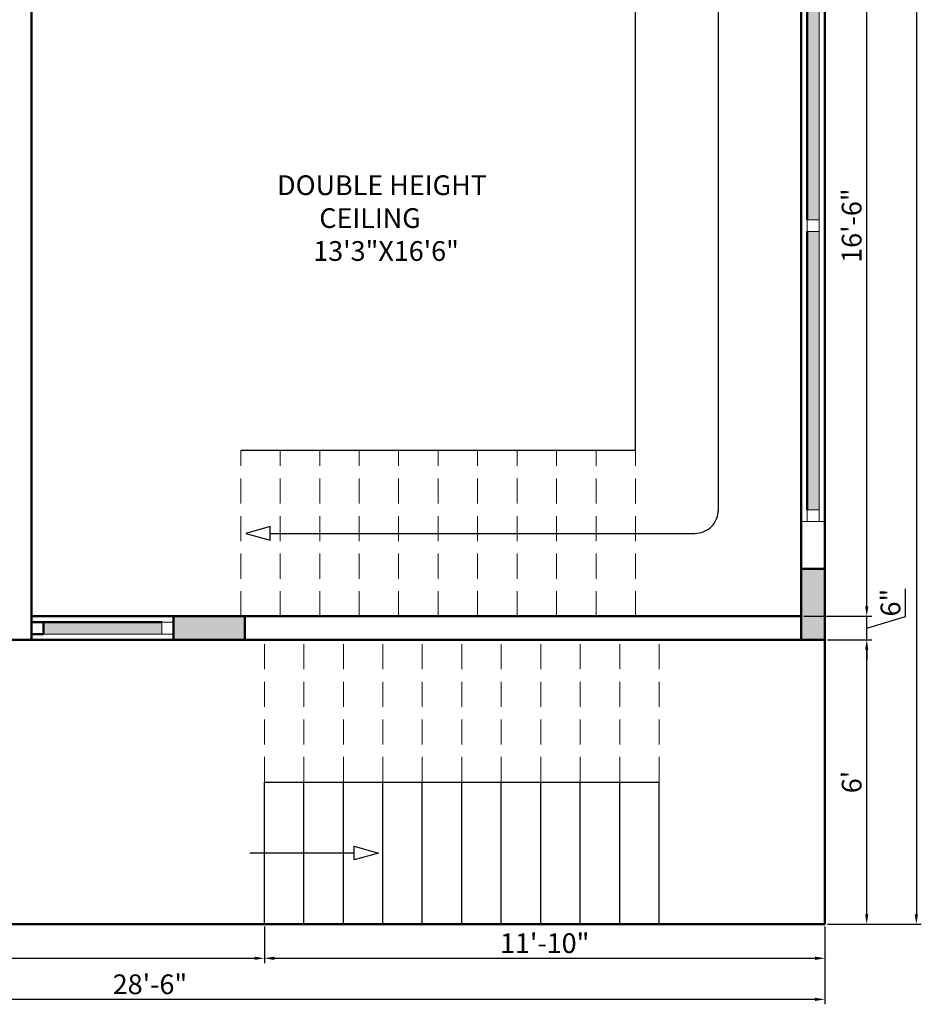
# Model space of a CAD drawing. Units: inches. Extents: x 3064 to 19385, y 846 to 15425.
# Tile 72 of 108: x 6607 to 6835, y 1476 to 1725. Entities that reach past the tile are written whole.
import ezdxf

# ---------------------------------------------------------------- set-up
doc = ezdxf.new("R2010")
doc.units = ezdxf.units.IN
doc.linetypes.add('DASHED', pattern=[19.05, 12.7, -6.35])
for name, color, linetype, lineweight in [('A-ANNO-DIMS', 2, 'Continuous', 18), ('A-AREA-IDEN', 3, 'Continuous', 18), ('A-COLS', 1, 'Continuous', 35), ('A-FLOR-STRS', 2, 'Continuous', 25), ('A-FLOR-STRS-OVHD', 2, 'DASHED', 18), ('A-GLAZ', 4, 'Continuous', 18), ('A-WALL', 7, 'Continuous', 50)]:
    doc.layers.add(name, color=color, linetype=linetype, lineweight=lineweight)
doc.styles.get("Standard").update_dxf_attribs({"font": 'arial.ttf'})
doc.dimstyles.new('ISO-25', dxfattribs={"dimtxt": 9, "dimasz": 2.5, "dimexe": 1.25, "dimexo": 0.625, "dimtad": 1, "dimdec": 1, "dimlunit": 3, "dimtxsty": 'Standard', "dimcen": 2.5, "dimadec": 0, "dimazin": 0, "dimtfac": 1, "dimtdec": 1, "dimtmove": 0, "dimatfit": 3, "dimfxl": 1, "dimarcsym": 0})

# ---------------------------------------------------------------- blocks, each defined once
blk = doc.blocks.new('*D359')
at = {"layer": 'A-ANNO-DIMS', "color": 0, "lineweight": -2, "transparency": 16777216}
for p, q in [((6469.03, 1495.36), (6469.03, 1486.07)), ((6669.03, 1495.36), (6669.03, 1486.07)), ((6471.53, 1487.32), (6666.53, 1487.32))]:
    blk.add_line(p, q, dxfattribs=at)
at = {"layer": 'A-ANNO-DIMS', "color": 0, "transparency": 16777216}
for points in [[(6471.53, 1487.73), (6471.53, 1486.9), (6469.03, 1487.32)], [(6666.53, 1487.73), (6666.53, 1486.9), (6669.03, 1487.32)]]:
    blk.add_solid(points, dxfattribs=at)
at = {"layer": 'Defpoints', "color": 0, "transparency": 16777216}
for p in [(6469.03, 1495.99), (6669.03, 1495.99), (6669.03, 1487.32)]:
    blk.add_point(p, dxfattribs=at)
at = {"layer": 'A-ANNO-DIMS', "color": 0, "transparency": 16777216, "insert": (6569.03, 1490.49), "char_height": 5, "attachment_point": 5}
blk.add_mtext('16\'-8"', dxfattribs=at)
blk = doc.blocks.new('*D360')
at = {"layer": 'A-ANNO-DIMS', "color": 0, "lineweight": -2, "transparency": 16777216}
for p, q in [((6669.03, 1495.36), (6669.03, 1486.07)), ((6811.03, 1495.36), (6811.03, 1486.07)), ((6671.53, 1487.32), (6808.53, 1487.32))]:
    blk.add_line(p, q, dxfattribs=at)
at = {"layer": 'A-ANNO-DIMS', "color": 0, "transparency": 16777216}
for points in [[(6671.53, 1487.73), (6671.53, 1486.9), (6669.03, 1487.32)], [(6808.53, 1487.73), (6808.53, 1486.9), (6811.03, 1487.32)]]:
    blk.add_solid(points, dxfattribs=at)
at = {"layer": 'Defpoints', "color": 0, "transparency": 16777216}
for p in [(6669.03, 1495.99), (6811.03, 1495.99), (6811.03, 1487.32)]:
    blk.add_point(p, dxfattribs=at)
at = {"layer": 'A-ANNO-DIMS', "color": 0, "transparency": 16777216, "insert": (6740.03, 1490.49), "char_height": 5, "attachment_point": 5}
blk.add_mtext('11\'-10"', dxfattribs=at)
blk = doc.blocks.new('*D342')
at = {"layer": 'A-ANNO-DIMS', "color": 0, "lineweight": -2, "transparency": 16777216}
for p, q in [((6469.03, 1495.36), (6469.03, 1475.66)), ((6811.03, 1495.36), (6811.03, 1475.66)), ((6808.53, 1476.91), (6471.53, 1476.91))]:
    blk.add_line(p, q, dxfattribs=at)
at = {"layer": 'A-ANNO-DIMS', "color": 0, "transparency": 16777216}
for points in [[(6471.53, 1477.32), (6471.53, 1476.49), (6469.03, 1476.91)], [(6808.53, 1477.32), (6808.53, 1476.49), (6811.03, 1476.91)]]:
    blk.add_solid(points, dxfattribs=at)
at = {"layer": 'Defpoints', "color": 0, "transparency": 16777216}
for p in [(6469.03, 1495.99), (6811.03, 1495.99), (6469.03, 1476.91)]:
    blk.add_point(p, dxfattribs=at)
at = {"layer": 'A-ANNO-DIMS', "color": 0, "transparency": 16777216, "insert": (6640.03, 1480.08), "char_height": 5, "attachment_point": 5}
blk.add_mtext('28\'-6"', dxfattribs=at)
blk = doc.blocks.new('*D361')
at = {"layer": 'A-ANNO-DIMS', "color": 0, "lineweight": -2, "transparency": 16777216}
for p, q in [((6811.66, 1567.99), (6822.87, 1567.99)), ((6821.62, 1498.49), (6821.62, 1565.49)), ((6811.66, 1495.99), (6822.87, 1495.99))]:
    blk.add_line(p, q, dxfattribs=at)
at = {"layer": 'A-ANNO-DIMS', "color": 0, "transparency": 16777216}
for points in [[(6821.2, 1565.49), (6822.03, 1565.49), (6821.62, 1567.99)], [(6821.2, 1498.49), (6822.03, 1498.49), (6821.62, 1495.99)]]:
    blk.add_solid(points, dxfattribs=at)
at = {"layer": 'Defpoints', "color": 0, "transparency": 16777216}
for p in [(6811.03, 1567.99), (6821.62, 1567.99), (6811.03, 1495.99)]:
    blk.add_point(p, dxfattribs=at)
at = {"layer": 'A-ANNO-DIMS', "color": 0, "transparency": 16777216, "insert": (6818.44, 1531.99), "char_height": 5, "attachment_point": 5, "rotation": 90}
blk.add_mtext("6'", dxfattribs=at)
blk = doc.blocks.new('*D362')
at = {"layer": 'A-ANNO-DIMS', "color": 0, "lineweight": -2, "transparency": 16777216}
for p, q in [((6831.46, 1573.94), (6831.46, 1580.97)), ((6821.62, 1576.49), (6821.62, 1578.99)), ((6805.66, 1573.99), (6822.87, 1573.99)), ((6821.62, 1567.99), (6821.62, 1573.99)), ((6821.62, 1567.99), (6821.62, 1573.99)), ((6821.62, 1570.99), (6831.46, 1573.94)), ((6811.66, 1567.99), (6822.87, 1567.99)), ((6821.62, 1565.49), (6821.62, 1562.99))]:
    blk.add_line(p, q, dxfattribs=at)
at = {"layer": 'A-ANNO-DIMS', "color": 0, "transparency": 16777216}
for points in [[(6821.2, 1576.49), (6822.03, 1576.49), (6821.62, 1573.99)], [(6821.2, 1565.49), (6822.03, 1565.49), (6821.62, 1567.99)]]:
    blk.add_solid(points, dxfattribs=at)
at = {"layer": 'Defpoints', "color": 0, "transparency": 16777216}
for p in [(6805.03, 1573.99), (6821.62, 1573.99), (6811.03, 1567.99)]:
    blk.add_point(p, dxfattribs=at)
at = {"layer": 'A-ANNO-DIMS', "color": 0, "transparency": 16777216, "insert": (6828.28, 1577.45), "char_height": 5, "attachment_point": 5, "rotation": 90}
blk.add_mtext('6"', dxfattribs=at)
blk = doc.blocks.new('*D363')
at = {"layer": 'A-ANNO-DIMS', "color": 0, "lineweight": -2, "transparency": 16777216}
for p, q in [((6811.66, 1771.99), (6822.87, 1771.99)), ((6821.62, 1576.49), (6821.62, 1769.49)), ((6805.66, 1573.99), (6822.87, 1573.99))]:
    blk.add_line(p, q, dxfattribs=at)
at = {"layer": 'A-ANNO-DIMS', "color": 0, "transparency": 16777216}
for points in [[(6821.2, 1769.49), (6822.03, 1769.49), (6821.62, 1771.99)], [(6821.2, 1576.49), (6822.03, 1576.49), (6821.62, 1573.99)]]:
    blk.add_solid(points, dxfattribs=at)
at = {"layer": 'Defpoints', "color": 0, "transparency": 16777216}
for p in [(6811.03, 1771.99), (6821.62, 1771.99), (6805.03, 1573.99)]:
    blk.add_point(p, dxfattribs=at)
at = {"layer": 'A-ANNO-DIMS', "color": 0, "transparency": 16777216, "insert": (6818.44, 1672.99), "char_height": 5, "attachment_point": 5, "rotation": 90}
blk.add_mtext('16\'-6"', dxfattribs=at)
blk = doc.blocks.new('*D348')
at = {"layer": 'A-ANNO-DIMS', "color": 0, "lineweight": -2, "transparency": 16777216}
for p, q in [((6811.66, 1987.99), (6835.44, 1987.99)), ((6834.19, 1985.49), (6834.19, 1498.49)), ((6811.66, 1495.99), (6835.44, 1495.99))]:
    blk.add_line(p, q, dxfattribs=at)
at = {"layer": 'A-ANNO-DIMS', "color": 0, "transparency": 16777216}
for points in [[(6833.77, 1985.49), (6834.6, 1985.49), (6834.19, 1987.99)], [(6833.77, 1498.49), (6834.6, 1498.49), (6834.19, 1495.99)]]:
    blk.add_solid(points, dxfattribs=at)
at = {"layer": 'Defpoints', "color": 0, "transparency": 16777216}
for p in [(6811.03, 1987.99), (6811.03, 1495.99), (6834.19, 1495.99)]:
    blk.add_point(p, dxfattribs=at)
at = {"layer": 'A-ANNO-DIMS', "color": 0, "transparency": 16777216, "insert": (6831.05, 1741.99), "char_height": 5, "attachment_point": 5, "rotation": 90}
blk.add_mtext("41'", dxfattribs=at)
blk = doc.blocks.new('WIN-1800-PAIR')
h = blk.add_hatch(color=256)
h.dxf.hatch_style = 1
h.paths.add_polyline_path([(0, 0), (3, 0), (3, 70.5), (0, 70.5)])
h.paths.add_polyline_path([(3, 144), (0, 144), (0, 73.5), (3, 73.5)])
blk.add_line((3, 144), (3, 73.5))
blk.add_lwpolyline([(3, 144), (0, 144), (0, 147), (3, 147)], close=True)
blk = doc.blocks.new('WIN-900')
blk.add_line((0, 0), (30, 0))
blk.add_lwpolyline([(30, 0), (30, 3), (33, 3), (33, 0)], close=True)
blk = doc.blocks.new('WIN-2000')
blk.add_line((3, 0), (3, 70.5))
blk.add_lwpolyline([(3, 70.5), (0, 70.5), (0, 73.5), (3, 73.5)], close=True)

msp = doc.modelspace()

# ---------------------------------------------------------------- hatches: boundary and pattern name
at = {"layer": 'A-COLS'}
h = msp.add_hatch(color=256, dxfattribs=at)
h.dxf.hatch_style = 1
h.paths.add_polyline_path([(6805.03, 1567.99), (6811.03, 1567.99), (6811.03, 1585.99), (6805.03, 1585.99)])
h = msp.add_hatch(color=256, dxfattribs=at)
h.dxf.hatch_style = 1
h.paths.add_polyline_path([(6664.03, 1567.99), (6664.03, 1573.99), (6646.03, 1573.99), (6646.03, 1567.99)])
at = {"layer": 'A-GLAZ'}
h = msp.add_hatch(color=256, dxfattribs=at)
h.dxf.hatch_style = 1
h.paths.add_polyline_path([(6613.03, 1572.49), (6613.03, 1569.49), (6643.03, 1569.49), (6643.03, 1572.49)])

# ---------------------------------------------------------------- linework, layer by layer
at = {"layer": 'A-FLOR-STRS'}
for p, q in [((6763.03, 1615.99), (6763.03, 1771.99)), ((6763.03, 1615.99), (6663.03, 1615.99)), ((6669.03, 1495.99), (6669.03, 1531.99)), ((6669.03, 1531.99), (6769.03, 1531.99)), ((6679.03, 1495.99), (6679.03, 1531.99)), ((6689.03, 1495.99), (6689.03, 1531.99)), ((6699.03, 1495.99), (6699.03, 1531.99)), ((6709.03, 1495.99), (6709.03, 1531.99)), ((6719.03, 1495.99), (6719.03, 1531.99)), ((6729.03, 1495.99), (6729.03, 1531.99)), ((6739.03, 1495.99), (6739.03, 1531.99)), ((6749.03, 1495.99), (6749.03, 1531.99)), ((6759.03, 1495.99), (6759.03, 1531.99)), ((6769.03, 1495.99), (6769.03, 1531.99)), ((6691.74, 1513.99), (6665.34, 1513.99))]:
    msp.add_line(p, q, dxfattribs=at)
msp.add_lwpolyline([(6670.52, 1594.99), (6778.03, 1594.99, 0.414214), (6784.03, 1600.99), (6784.03, 1744.99, 0.414214), (6778.03, 1750.99), (6651.03, 1750.99)], format="xyb", dxfattribs=at)
for points in [[(6664.33, 1594.99), (6670.52, 1593.26), (6670.52, 1596.72)], [(6697.93, 1513.99), (6691.74, 1512.26), (6691.74, 1515.72)]]:
    msp.add_lwpolyline(points, close=True, dxfattribs=at)
at = {"layer": 'A-FLOR-STRS-OVHD', "ltscale": 0.5}
for p, q in [((6663.03, 1573.99), (6663.03, 1615.99)), ((6673.03, 1573.99), (6673.03, 1615.99)), ((6683.03, 1573.99), (6683.03, 1615.99)), ((6693.03, 1573.99), (6693.03, 1615.99)), ((6703.03, 1573.99), (6703.03, 1615.99)), ((6713.03, 1573.99), (6713.03, 1615.99)), ((6723.03, 1573.99), (6723.03, 1615.99)), ((6733.03, 1573.99), (6733.03, 1615.99)), ((6743.03, 1573.99), (6743.03, 1615.99)), ((6753.03, 1573.99), (6753.03, 1615.99)), ((6763.03, 1573.99), (6763.03, 1615.99)), ((6669.03, 1531.99), (6669.03, 1567.99)), ((6679.03, 1531.99), (6679.03, 1567.99)), ((6689.03, 1531.99), (6689.03, 1567.99)), ((6699.03, 1531.99), (6699.03, 1567.99)), ((6709.03, 1531.99), (6709.03, 1567.99)), ((6719.03, 1531.99), (6719.03, 1567.99)), ((6729.03, 1531.99), (6729.03, 1567.99)), ((6739.03, 1531.99), (6739.03, 1567.99)), ((6749.03, 1531.99), (6749.03, 1567.99)), ((6759.03, 1531.99), (6759.03, 1567.99)), ((6769.03, 1531.99), (6769.03, 1567.99))]:
    msp.add_line(p, q, dxfattribs=at)
at = {"layer": 'A-GLAZ'}
msp.add_line((6811.03, 1597.99), (6805.03, 1597.99), dxfattribs=at)
msp.add_line((6811.03, 1597.99), (6805.03, 1597.99), dxfattribs=at)
msp.add_lwpolyline([(6809.53, 1597.99), (6806.53, 1597.99), (6806.53, 1600.99), (6809.53, 1600.99)], close=True, dxfattribs=at)
at = {"layer": 'A-WALL'}
for p, q in [((6811.03, 1495.99), (6811.03, 1987.99)), ((6805.03, 1573.99), (6805.03, 1771.99)), ((6806.53, 1744.99), (6806.53, 1674.49)), ((6610.03, 1735.99), (6610.03, 1567.99)), ((6806.53, 1600.99), (6806.53, 1671.49)), ((6805.03, 1573.99), (6610.03, 1573.99)), ((6610.03, 1567.99), (6610.03, 1573.99)), ((6613.03, 1572.49), (6643.03, 1572.49)), ((6646.03, 1567.99), (6646.03, 1573.99)), ((6646.03, 1567.99), (6646.03, 1573.99)), ((6811.03, 1567.99), (6469.03, 1567.99)), ((6469.03, 1495.99), (6811.03, 1495.99))]:
    msp.add_line(p, q, dxfattribs=at)
for points in [[(6811.03, 1567.99), (6811.03, 1585.99), (6805.03, 1585.99), (6805.03, 1567.99)], [(6610.03, 1569.49), (6610.03, 1572.49), (6613.03, 1572.49), (6613.03, 1569.49)], [(6664.03, 1573.99), (6646.03, 1573.99), (6646.03, 1567.99), (6664.03, 1567.99)]]:
    msp.add_lwpolyline(points, close=True, dxfattribs=at)

# ---------------------------------------------------------------- block references
at = {"layer": 'A-GLAZ'}
for name, p in [('WIN-1800-PAIR', (6806.53, 1600.99)), ('WIN-2000', (6806.53, 1600.99)), ('WIN-900', (6613.03, 1569.49))]:
    msp.add_blockref(name, p, dxfattribs=at)

# ---------------------------------------------------------------- texts
at = {"layer": 'A-AREA-IDEN', "insert": (6672.24, 1685.72), "char_height": 5, "attachment_point": 1}
msp.add_mtext_dynamic_manual_height_columns('DOUBLE HEIGHT \\P       CEILING            \\P      13\'3"X16\'6"', width=57.0817, gutter_width=12.5, heights=[0], dxfattribs=at)

# ---------------------------------------------------------------- dimensions: what is measured, and where the dimension line sits
at = {"layer": 'A-ANNO-DIMS'}
for base, p1, p2, override, picture, middle in [((6834.19, 1495.99), (6811.03, 1987.99), (6811.03, 1495.99), {"dimtxt": 5, "dimclrd": 0, "dimclre": 0, "dimclrt": 0}, '*D348', (6831.05, 1741.99)), ((6821.62, 1771.99), (6805.03, 1573.99), (6811.03, 1771.99), {"dimtxt": 5, "dimclrd": 0, "dimclre": 0, "dimclrt": 0, "dimtmove": 1}, '*D363', (6818.44, 1672.99)), ((6821.62, 1573.99), (6811.03, 1567.99), (6805.03, 1573.99), {"dimtxt": 5, "dimclrd": 0, "dimclre": 0, "dimclrt": 0, "dimtmove": 1}, '*D362', (6828.28, 1574.57)), ((6821.62, 1567.99), (6811.03, 1495.99), (6811.03, 1567.99), {"dimtxt": 5, "dimclrd": 0, "dimclre": 0, "dimclrt": 0}, '*D361', (6818.44, 1531.99))]:
    dim = msp.add_linear_dim(base=base, p1=p1, p2=p2, angle=90, dimstyle='ISO-25', override=override, dxfattribs=at)
    dim.commit()
    dim.dimension.update_dxf_attribs({"geometry": picture, "text_midpoint": middle})
for base, p1, p2, override, picture, middle in [((6669.03, 1487.32), (6469.03, 1495.99), (6669.03, 1495.99), {"dimtxt": 5, "dimclrd": 0, "dimclre": 0, "dimclrt": 0}, '*D359', (6569.03, 1490.49)), ((6469.03, 1476.91), (6811.03, 1495.99), (6469.03, 1495.99), {"dimtxt": 5, "dimclrd": 0, "dimclre": 0, "dimclrt": 0}, '*D342', (6640.03, 1480.08)), ((6811.03, 1487.32), (6669.03, 1495.99), (6811.03, 1495.99), {"dimtxt": 5, "dimclrd": 0, "dimclre": 0, "dimclrt": 0, "dimtmove": 1}, '*D360', (6740.03, 1490.49))]:
    dim = msp.add_linear_dim(base=base, p1=p1, p2=p2, dimstyle='ISO-25', override=override, dxfattribs=at)
    dim.commit()
    dim.dimension.update_dxf_attribs({"geometry": picture, "text_midpoint": middle})

doc.saveas('drawing.dxf')
